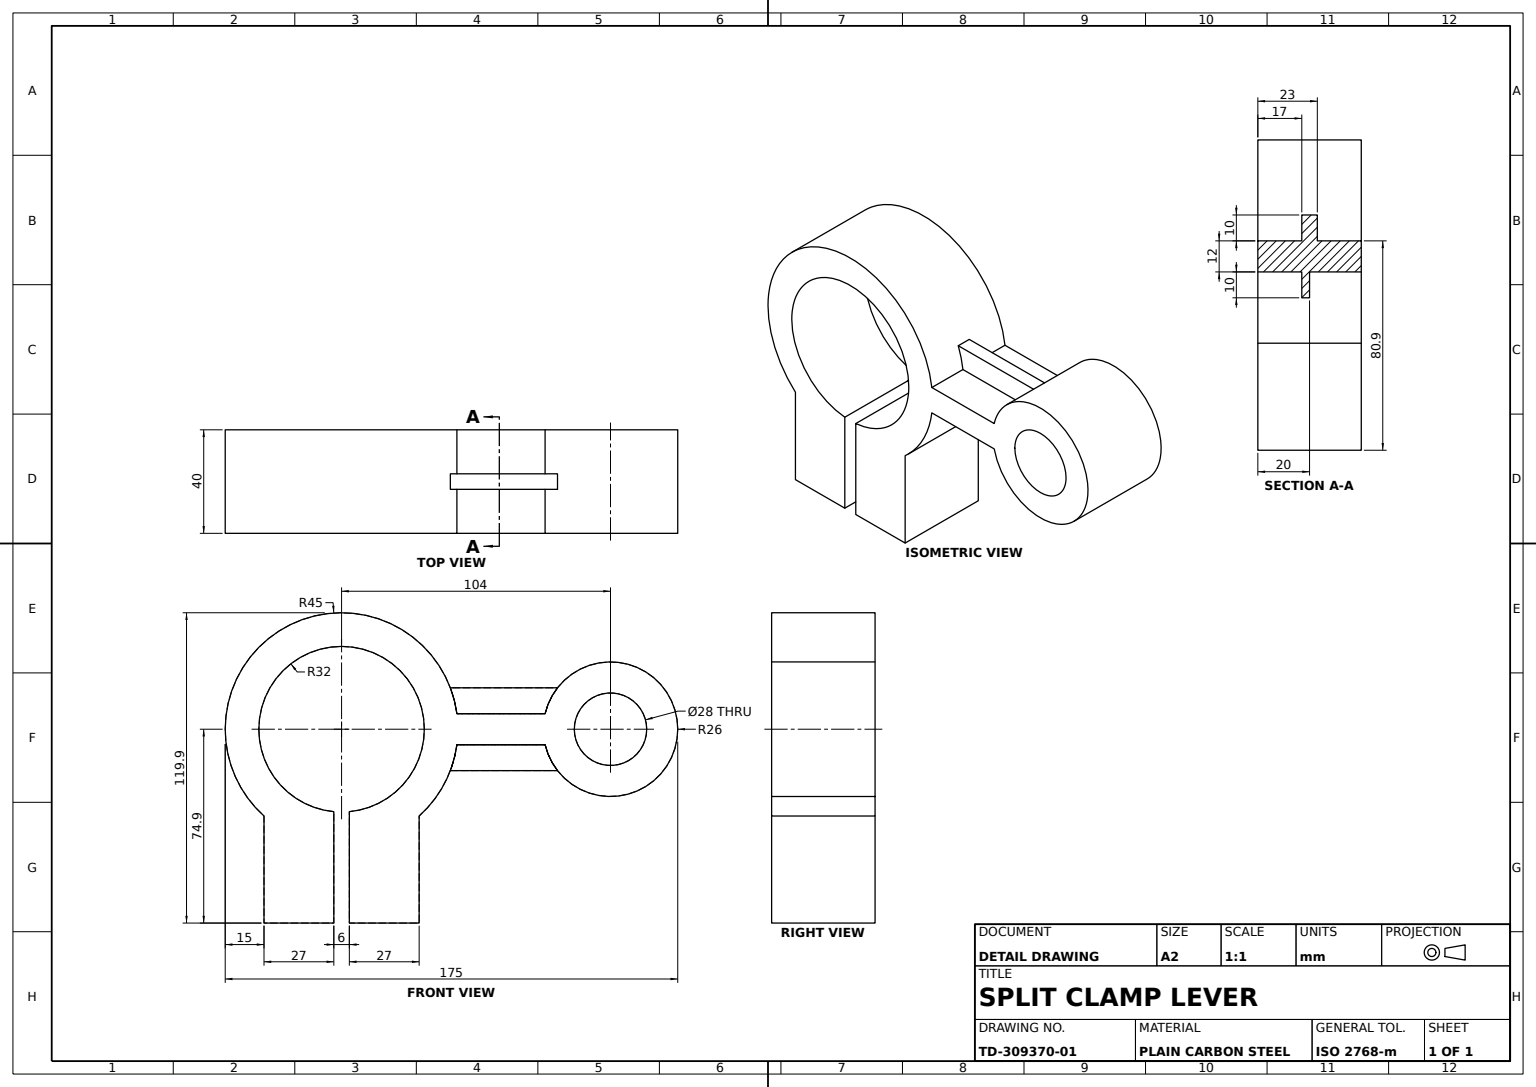
from build123d import *

# Parameters (mm, degrees)
CLAMP_BODY_DEPTH             = 40
PIN_BORE_SKETCH_R            = 14
PIN_BORE_28_DEPTH            = 40
CLAMP_START                  = -40
CLAMP_BORE_64_AND_SLIT_DEPTH = 40
LEVER_START                  = -40
LEVER_ARM_DEPTH              = 40
ARM_WEB_A_DEPTH              = 10
ARM_WEB_B_DEPTH              = 10


with BuildPart() as part:
    # Clamp Body Sketch → Clamp Body (new body)
    with BuildSketch(Plane.XY):
        with BuildLine():
            Line((52, -6), (78.701778719, -6))
            ThreePointArc((78.701778719, -6), (130, 0), (78.701778719, 6))
            Line((78.701778719, 6), (52, 6))
            Line((52, 6), (44.598206242, 6))
            ThreePointArc((44.598206242, 6), (-45, 0), (44.598206242, -6))
            Line((44.598206242, -6), (52, -6))
        make_face()
    extrude(amount=CLAMP_BODY_DEPTH)

    # Pin Bore Sketch → Pin Bore Ø28 (cut)
    with BuildSketch(Plane.XY.offset(40)):
        with Locations((104, 0)):
            Circle(PIN_BORE_SKETCH_R)
    extrude(amount=-PIN_BORE_28_DEPTH, mode=Mode.SUBTRACT)

    # Clamp Bore and Slit Sketch → Clamp Bore Ø64 and Slit (cut)
    with BuildSketch(Plane.XY.offset(40).offset(CLAMP_START)):
        with BuildLine():
            ThreePointArc((-3, -44.899888641), (0, -45), (3, -44.899888641))
            Line((3, -44.899888641), (3, -31.859064644))
            ThreePointArc((3, -31.859064644), (19.483742845, -25.38471518), (30, -11.135528726))
            ThreePointArc((30, -11.135528726), (0, 32), (-30, -11.135528726))
            ThreePointArc((-30, -11.135528726), (-19.483742845, -25.38471518), (-3, -31.859064644))
            Line((-3, -31.859064644), (-3, -44.899888641))
        make_face()
    extrude(amount=CLAMP_BORE_64_AND_SLIT_DEPTH, mode=Mode.SUBTRACT)

    # Lever Arm Sketch → Lever Arm (add)
    with BuildSketch(Plane.XY.offset(40).offset(LEVER_START)):
        with BuildLine():
            Line((-3, -44.899888641), (-3, -74.899888641))
            Line((-3, -74.899888641), (-30, -74.899888641))
            Line((-30, -74.899888641), (-30, -33.541019662))
            ThreePointArc((-30, -33.541019662), (-17.450099602, -41.478838266), (-3, -44.899888641))
        make_face()
        with BuildLine():
            Line((3, -44.899888641), (3, -74.899888641))
            Line((3, -74.899888641), (30, -74.899888641))
            Line((30, -74.899888641), (30, -33.541019662))
            ThreePointArc((30, -33.541019662), (17.450099602, -41.478838266), (3, -44.899888641))
        make_face()
    extrude(amount=LEVER_ARM_DEPTH)

    # Arm Web A Sketch → Arm Web A (add)
    with BuildSketch(Plane(origin=(0, 6, 0), x_dir=(1, 0, 0), z_dir=(0, 1, 0))):
        Polygon((32.912600582, -20), (32.912600582, -17), (88.947224008, -17), (88.947224008, -23), (32.912600582, -23), align=None)
    extrude(amount=ARM_WEB_A_DEPTH)

    # Arm Web B Sketch → Arm Web B (add)
    with BuildSketch(Plane.XZ.offset(6)):
        Polygon((44.598206242, 23), (37.493332774, 23), (37.493332774, 20), (86.340481081, 20), (86.340481081, 23), align=None)
    extrude(amount=ARM_WEB_B_DEPTH)


solid = part.part
